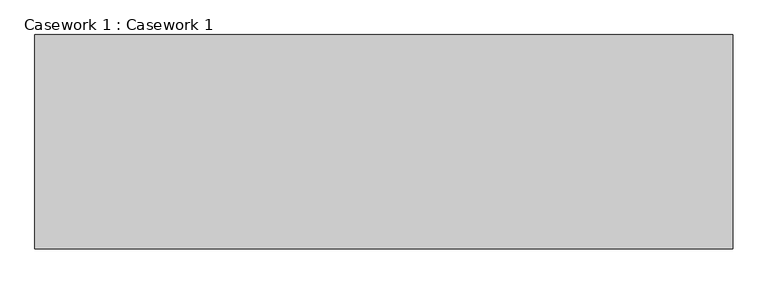
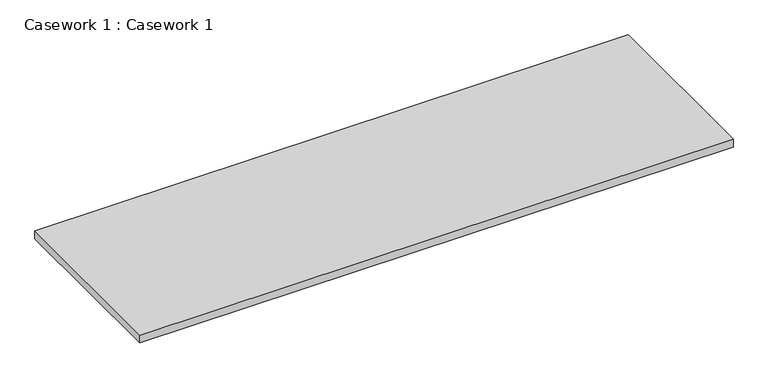
"""IFC4 building model written with IfcOpenShell, lengths in millimetres: furniture geometry, Casework 1 : Casework 1."""

from ifc_helpers import new_model, si_unit, frame, origin, place, context, project, spatial, polyline, outline, extrude, source, transform, mapped, element, save


def casework_1_casework_1_edaa4522(model_context):
    return source(origin(), model_context, "Body", "SweptSolid", [
        extrude(outline(polyline([(627.2834347, 5642.1857557), (627.2834347, 4956.3857557), (-1607.9165653, 4956.3857557), (-1607.9165653, 5642.1857557), (627.2834347, 5642.1857557)])), frame((0.0, 0.0, 1070.3966031), z_axis=(0.0, 0.0, 1.0), x_axis=(1.0, 0.0, 0.0)), (0.0, 0.0, 1.0), 30.7470961),
    ])


if __name__ == "__main__":
    model = new_model("IFC4")
    model_context = context("Model", 3, world=origin())
    ifc_project = project(units=[si_unit("LENGTHUNIT", "METRE", prefix="MILLI")], contexts=[model_context])
    site = spatial("IfcSite", under=ifc_project)
    building = spatial("IfcBuilding", under=site)
    placement = place(None, origin())
    casework_1_casework_1_shape = casework_1_casework_1_edaa4522(model_context)
    element("IfcFurniture", 1, ObjectType="Casework 1 : Casework 1", at=placement, inside=building, context=model_context, shape_type="MappedRepresentation", body=[
        mapped(casework_1_casework_1_shape, transform((0.0, 0.0, 0.0), x_axis=(1.0, 0.0, 0.0), y_axis=(0.0, 1.0, 0.0), z_axis=(0.0, 0.0, 1.0))),
    ])
    save(model, "model.ifc")
